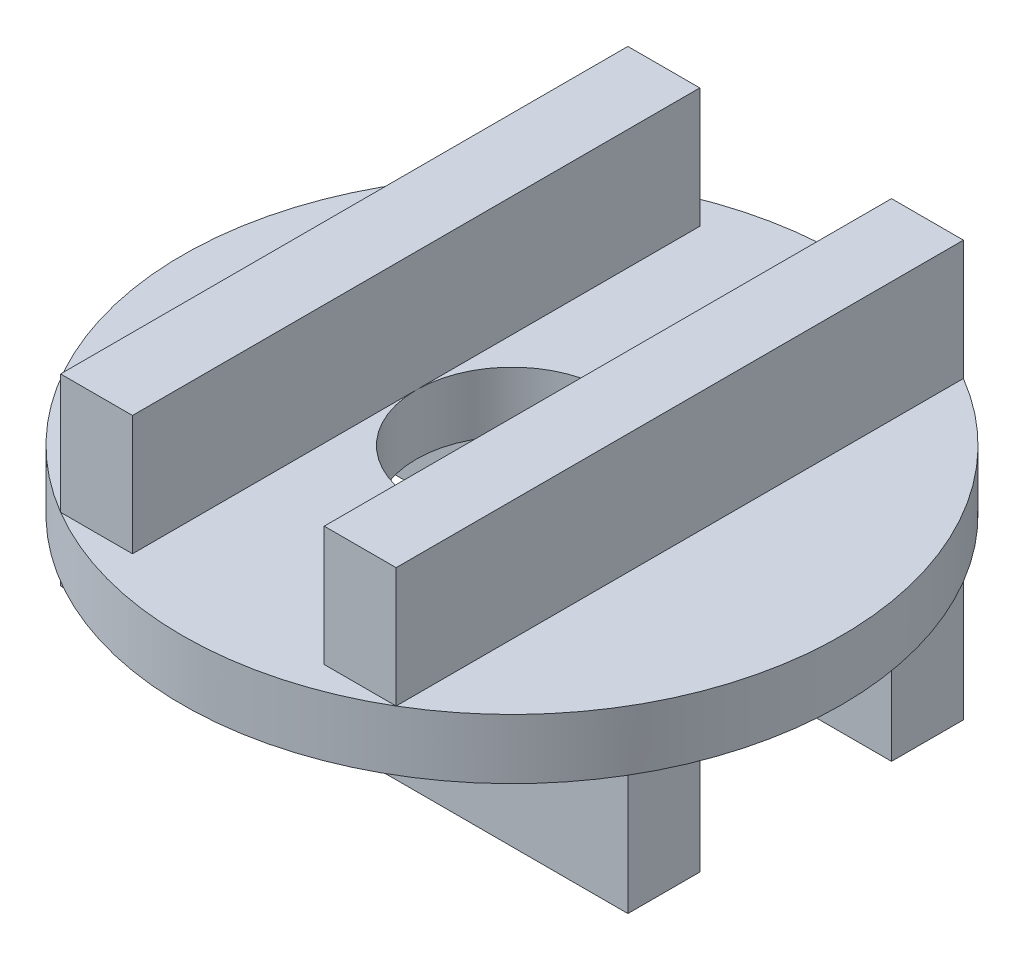
ISO-10303-21;
HEADER;
FILE_DESCRIPTION(('STEP AP214'),'2;1');
FILE_NAME('part.step','',(''),(''),'','','');
FILE_SCHEMA(('AUTOMOTIVE_DESIGN { 1 0 10303 214 1 1 1 1 }'));
ENDSEC;
DATA;
#1=APPLICATION_CONTEXT('core data for automotive mechanical design processes');
#2=APPLICATION_PROTOCOL_DEFINITION('international standard','automotive_design',2000,#1);
#3=PRODUCT_CONTEXT('',#1,'mechanical');
#4=PRODUCT('Part','Part','',(#3));
#5=PRODUCT_RELATED_PRODUCT_CATEGORY('part','',(#4));
#6=PRODUCT_DEFINITION_FORMATION('','',#4);
#7=PRODUCT_DEFINITION_CONTEXT('part definition',#1,'design');
#8=PRODUCT_DEFINITION('design','',#6,#7);
#9=PRODUCT_DEFINITION_SHAPE('','',#8);
#10=(LENGTH_UNIT() NAMED_UNIT(*) SI_UNIT(.MILLI.,.METRE.));
#11=(NAMED_UNIT(*) PLANE_ANGLE_UNIT() SI_UNIT($,.RADIAN.));
#12=(NAMED_UNIT(*) SI_UNIT($,.STERADIAN.) SOLID_ANGLE_UNIT());
#13=UNCERTAINTY_MEASURE_WITH_UNIT(LENGTH_MEASURE(1.E-05),#10,'distance_accuracy_value','');
#14=(GEOMETRIC_REPRESENTATION_CONTEXT(3) GLOBAL_UNCERTAINTY_ASSIGNED_CONTEXT((#13)) GLOBAL_UNIT_ASSIGNED_CONTEXT((#10,
#11,#12)) REPRESENTATION_CONTEXT('',''));
#15=CARTESIAN_POINT('',(0.,0.,0.));
#16=DIRECTION('',(0.,0.,1.));
#17=DIRECTION('',(1.,0.,0.));
#18=AXIS2_PLACEMENT_3D('',#15,#16,#17);
#19=CARTESIAN_POINT('',(0.,0.,0.));
#20=DIRECTION('',(0.,1.,0.));
#21=DIRECTION('',(0.,0.,1.));
#22=AXIS2_PLACEMENT_3D('',#19,#20,#21);
#23=PLANE('',#22);
#24=DIRECTION('',(0.,0.,1.));
#25=VECTOR('',#24,1.);
#26=CARTESIAN_POINT('',(47.3392015141785,0.,1.64240848401284E-13));
#27=LINE('',#26,#25);
#28=CARTESIAN_POINT('',(47.3392015141785,0.,16.0000000000002));
#29=VERTEX_POINT('',#28);
#30=CARTESIAN_POINT('',(47.3392015141784,0.,28.0000000000002));
#31=VERTEX_POINT('',#30);
#32=EDGE_CURVE('E70',#29,#31,#27,.T.);
#33=ORIENTED_EDGE('',*,*,#32,.F.);
#34=DIRECTION('',(-1.,0.,0.));
#35=VECTOR('',#34,1.);
#36=CARTESIAN_POINT('',(0.,0.,16.));
#37=LINE('',#36,#35);
#38=CARTESIAN_POINT('',(0.,0.,16.));
#39=VERTEX_POINT('',#38);
#40=EDGE_CURVE('E53',#29,#39,#37,.T.);
#41=ORIENTED_EDGE('',*,*,#40,.T.);
#42=CARTESIAN_POINT('',(0.,0.,0.));
#43=DIRECTION('',(0.,1.,0.));
#44=DIRECTION('',(0.,0.,1.));
#45=AXIS2_PLACEMENT_3D('',#42,#43,#44);
#46=CIRCLE('',#45,16.);
#47=CARTESIAN_POINT('',(0.,0.,-16.));
#48=VERTEX_POINT('',#47);
#49=EDGE_CURVE('E313',#39,#48,#46,.T.);
#50=ORIENTED_EDGE('',*,*,#49,.T.);
#51=DIRECTION('',(-1.,0.,0.));
#52=VECTOR('',#51,1.);
#53=CARTESIAN_POINT('',(0.,0.,-16.));
#54=LINE('',#53,#52);
#55=CARTESIAN_POINT('',(47.3392015141786,0.,-15.9999999999998));
#56=VERTEX_POINT('',#55);
#57=EDGE_CURVE('E228',#56,#48,#54,.T.);
#58=ORIENTED_EDGE('',*,*,#57,.F.);
#59=DIRECTION('',(0.,0.,-1.));
#60=VECTOR('',#59,1.);
#61=CARTESIAN_POINT('',(47.3392015141785,0.,1.64240848401285E-13));
#62=LINE('',#61,#60);
#63=CARTESIAN_POINT('',(47.3392015141786,0.,-27.9999999999998));
#64=VERTEX_POINT('',#63);
#65=EDGE_CURVE('E224',#56,#64,#62,.T.);
#66=ORIENTED_EDGE('',*,*,#65,.T.);
#67=CARTESIAN_POINT('',(0.,0.,0.));
#68=DIRECTION('',(0.,1.,0.));
#69=DIRECTION('',(0.,0.,1.));
#70=AXIS2_PLACEMENT_3D('',#67,#68,#69);
#71=CIRCLE('',#70,55.);
#72=EDGE_CURVE('E50',#31,#64,#71,.T.);
#73=ORIENTED_EDGE('',*,*,#72,.F.);
#74=EDGE_LOOP('',(#33,#41,#50,#58,#66,#73));
#75=FACE_BOUND('',#74,.T.);
#76=ADVANCED_FACE('F43',(#75),#23,.F.);
#77=DIRECTION('',(-1.,0.,0.));
#78=VECTOR('',#77,1.);
#79=CARTESIAN_POINT('',(0.,0.,28.));
#80=LINE('',#79,#78);
#81=CARTESIAN_POINT('',(-47.3392015141786,0.,27.9999999999998));
#82=VERTEX_POINT('',#81);
#83=EDGE_CURVE('E193',#31,#82,#80,.T.);
#84=ORIENTED_EDGE('',*,*,#83,.F.);
#85=EDGE_CURVE('E310',#82,#31,#71,.T.);
#86=ORIENTED_EDGE('',*,*,#85,.F.);
#87=EDGE_LOOP('',(#84,#86));
#88=FACE_BOUND('',#87,.T.);
#89=ADVANCED_FACE('F341',(#88),#23,.F.);
#90=EDGE_CURVE('E272',#48,#39,#46,.T.);
#91=ORIENTED_EDGE('',*,*,#90,.T.);
#92=CARTESIAN_POINT('',(-47.3392015141786,0.,15.9999999999998));
#93=VERTEX_POINT('',#92);
#94=EDGE_CURVE('E11',#39,#93,#37,.T.);
#95=ORIENTED_EDGE('',*,*,#94,.T.);
#96=DIRECTION('',(0.,0.,1.));
#97=VECTOR('',#96,1.);
#98=CARTESIAN_POINT('',(-47.3392015141785,0.,-1.64240848401284E-13));
#99=LINE('',#98,#97);
#100=EDGE_CURVE('E192',#93,#82,#99,.T.);
#101=ORIENTED_EDGE('',*,*,#100,.T.);
#102=CARTESIAN_POINT('',(-47.3392015141784,0.,-28.0000000000002));
#103=VERTEX_POINT('',#102);
#104=EDGE_CURVE('E332',#103,#82,#71,.T.);
#105=ORIENTED_EDGE('',*,*,#104,.F.);
#106=DIRECTION('',(0.,0.,-1.));
#107=VECTOR('',#106,1.);
#108=CARTESIAN_POINT('',(-47.3392015141785,0.,-1.91614323134832E-13));
#109=LINE('',#108,#107);
#110=CARTESIAN_POINT('',(-47.3392015141785,0.,-16.0000000000002));
#111=VERTEX_POINT('',#110);
#112=EDGE_CURVE('E215',#111,#103,#109,.T.);
#113=ORIENTED_EDGE('',*,*,#112,.F.);
#114=EDGE_CURVE('E55',#48,#111,#54,.T.);
#115=ORIENTED_EDGE('',*,*,#114,.F.);
#116=EDGE_LOOP('',(#91,#95,#101,#105,#113,#115));
#117=FACE_BOUND('',#116,.T.);
#118=ADVANCED_FACE('F350',(#117),#23,.F.);
#119=CARTESIAN_POINT('',(0.,10.,0.));
#120=DIRECTION('',(0.,1.,0.));
#121=DIRECTION('',(0.,0.,1.));
#122=AXIS2_PLACEMENT_3D('',#119,#120,#121);
#123=PLANE('',#122);
#124=DIRECTION('',(0.,0.,1.));
#125=VECTOR('',#124,1.);
#126=CARTESIAN_POINT('',(16.,10.,47.3392015141785));
#127=LINE('',#126,#125);
#128=CARTESIAN_POINT('',(16.,10.,0.));
#129=VERTEX_POINT('',#128);
#130=CARTESIAN_POINT('',(16.,10.,47.3392015141785));
#131=VERTEX_POINT('',#130);
#132=EDGE_CURVE('E261',#129,#131,#127,.T.);
#133=ORIENTED_EDGE('',*,*,#132,.F.);
#134=CARTESIAN_POINT('',(0.,10.,0.));
#135=DIRECTION('',(0.,1.,0.));
#136=DIRECTION('',(0.,0.,1.));
#137=AXIS2_PLACEMENT_3D('',#134,#135,#136);
#138=CIRCLE('',#137,16.);
#139=CARTESIAN_POINT('',(-16.,10.,0.));
#140=VERTEX_POINT('',#139);
#141=EDGE_CURVE('E309',#140,#129,#138,.T.);
#142=ORIENTED_EDGE('',*,*,#141,.F.);
#143=DIRECTION('',(0.,0.,-1.));
#144=VECTOR('',#143,1.);
#145=CARTESIAN_POINT('',(-16.,10.,47.3392015141785));
#146=LINE('',#145,#144);
#147=CARTESIAN_POINT('',(-16.,10.,47.3392015141785));
#148=VERTEX_POINT('',#147);
#149=EDGE_CURVE('E289',#148,#140,#146,.T.);
#150=ORIENTED_EDGE('',*,*,#149,.F.);
#151=DIRECTION('',(1.,0.,0.));
#152=VECTOR('',#151,1.);
#153=CARTESIAN_POINT('',(-16.,10.,47.3392015141785));
#154=LINE('',#153,#152);
#155=CARTESIAN_POINT('',(-28.,10.,47.3392015141785));
#156=VERTEX_POINT('',#155);
#157=EDGE_CURVE('E291',#156,#148,#154,.T.);
#158=ORIENTED_EDGE('',*,*,#157,.F.);
#159=CARTESIAN_POINT('',(0.,10.,0.));
#160=DIRECTION('',(0.,1.,0.));
#161=DIRECTION('',(0.,0.,1.));
#162=AXIS2_PLACEMENT_3D('',#159,#160,#161);
#163=CIRCLE('',#162,55.);
#164=CARTESIAN_POINT('',(28.,10.,47.3392015141785));
#165=VERTEX_POINT('',#164);
#166=EDGE_CURVE('E312',#156,#165,#163,.T.);
#167=ORIENTED_EDGE('',*,*,#166,.T.);
#168=DIRECTION('',(1.,0.,0.));
#169=VECTOR('',#168,1.);
#170=CARTESIAN_POINT('',(16.,10.,47.3392015141785));
#171=LINE('',#170,#169);
#172=EDGE_CURVE('E249',#131,#165,#171,.T.);
#173=ORIENTED_EDGE('',*,*,#172,.F.);
#174=EDGE_LOOP('',(#133,#142,#150,#158,#167,#173));
#175=FACE_BOUND('',#174,.T.);
#176=ADVANCED_FACE('F355',(#175),#123,.T.);
#177=CARTESIAN_POINT('',(16.,10.,-47.3392015141785));
#178=VERTEX_POINT('',#177);
#179=EDGE_CURVE('E245',#178,#129,#127,.T.);
#180=ORIENTED_EDGE('',*,*,#179,.F.);
#181=DIRECTION('',(-1.,0.,0.));
#182=VECTOR('',#181,1.);
#183=CARTESIAN_POINT('',(16.,10.,-47.3392015141785));
#184=LINE('',#183,#182);
#185=CARTESIAN_POINT('',(28.,10.,-47.3392015141785));
#186=VERTEX_POINT('',#185);
#187=EDGE_CURVE('E258',#186,#178,#184,.T.);
#188=ORIENTED_EDGE('',*,*,#187,.F.);
#189=CARTESIAN_POINT('',(-28.,10.,-47.3392015141785));
#190=VERTEX_POINT('',#189);
#191=EDGE_CURVE('E314',#186,#190,#163,.T.);
#192=ORIENTED_EDGE('',*,*,#191,.T.);
#193=DIRECTION('',(-1.,0.,0.));
#194=VECTOR('',#193,1.);
#195=CARTESIAN_POINT('',(-16.,10.,-47.3392015141785));
#196=LINE('',#195,#194);
#197=CARTESIAN_POINT('',(-16.,10.,-47.3392015141785));
#198=VERTEX_POINT('',#197);
#199=EDGE_CURVE('E287',#198,#190,#196,.T.);
#200=ORIENTED_EDGE('',*,*,#199,.F.);
#201=EDGE_CURVE('E294',#140,#198,#146,.T.);
#202=ORIENTED_EDGE('',*,*,#201,.F.);
#203=EDGE_CURVE('E308',#129,#140,#138,.T.);
#204=ORIENTED_EDGE('',*,*,#203,.F.);
#205=EDGE_LOOP('',(#180,#188,#192,#200,#202,#204));
#206=FACE_BOUND('',#205,.T.);
#207=ADVANCED_FACE('F589',(#206),#123,.T.);
#208=DIRECTION('',(0.,0.,-1.));
#209=VECTOR('',#208,1.);
#210=CARTESIAN_POINT('',(28.,10.,47.3392015141785));
#211=LINE('',#210,#209);
#212=EDGE_CURVE('E252',#165,#186,#211,.T.);
#213=ORIENTED_EDGE('',*,*,#212,.F.);
#214=EDGE_CURVE('E311',#165,#186,#163,.T.);
#215=ORIENTED_EDGE('',*,*,#214,.T.);
#216=EDGE_LOOP('',(#213,#215));
#217=FACE_BOUND('',#216,.T.);
#218=ADVANCED_FACE('F356',(#217),#123,.T.);
#219=DIRECTION('',(0.,0.,1.));
#220=VECTOR('',#219,1.);
#221=CARTESIAN_POINT('',(-28.,10.,47.3392015141785));
#222=LINE('',#221,#220);
#223=EDGE_CURVE('E251',#190,#156,#222,.T.);
#224=ORIENTED_EDGE('',*,*,#223,.F.);
#225=EDGE_CURVE('E321',#190,#156,#163,.T.);
#226=ORIENTED_EDGE('',*,*,#225,.T.);
#227=EDGE_LOOP('',(#224,#226));
#228=FACE_BOUND('',#227,.T.);
#229=ADVANCED_FACE('F357',(#228),#123,.T.);
#230=EDGE_CURVE('E330',#64,#103,#71,.T.);
#231=ORIENTED_EDGE('',*,*,#230,.F.);
#232=DIRECTION('',(-1.,0.,0.));
#233=VECTOR('',#232,1.);
#234=CARTESIAN_POINT('',(0.,0.,-28.));
#235=LINE('',#234,#233);
#236=EDGE_CURVE('E219',#64,#103,#235,.T.);
#237=ORIENTED_EDGE('',*,*,#236,.T.);
#238=EDGE_LOOP('',(#231,#237));
#239=FACE_BOUND('',#238,.T.);
#240=ADVANCED_FACE('F351',(#239),#23,.F.);
#241=CARTESIAN_POINT('',(0.,10.,0.));
#242=DIRECTION('',(0.,-1.,0.));
#243=DIRECTION('',(0.,0.,-1.));
#244=AXIS2_PLACEMENT_3D('',#241,#242,#243);
#245=CYLINDRICAL_SURFACE('',#244,55.);
#246=ORIENTED_EDGE('',*,*,#214,.F.);
#247=ORIENTED_EDGE('',*,*,#166,.F.);
#248=ORIENTED_EDGE('',*,*,#225,.F.);
#249=ORIENTED_EDGE('',*,*,#191,.F.);
#250=EDGE_LOOP('',(#246,#247,#248,#249));
#251=FACE_BOUND('',#250,.T.);
#252=ORIENTED_EDGE('',*,*,#72,.T.);
#253=ORIENTED_EDGE('',*,*,#230,.T.);
#254=ORIENTED_EDGE('',*,*,#104,.T.);
#255=ORIENTED_EDGE('',*,*,#85,.T.);
#256=EDGE_LOOP('',(#252,#253,#254,#255));
#257=FACE_BOUND('',#256,.T.);
#258=ADVANCED_FACE('F44',(#251,#257),#245,.T.);
#259=CARTESIAN_POINT('',(0.,10.,0.));
#260=DIRECTION('',(0.,-1.,0.));
#261=DIRECTION('',(0.,0.,-1.));
#262=AXIS2_PLACEMENT_3D('',#259,#260,#261);
#263=CYLINDRICAL_SURFACE('',#262,16.);
#264=ORIENTED_EDGE('',*,*,#203,.T.);
#265=ORIENTED_EDGE('',*,*,#141,.T.);
#266=EDGE_LOOP('',(#264,#265));
#267=FACE_BOUND('',#266,.T.);
#268=ORIENTED_EDGE('',*,*,#49,.F.);
#269=ORIENTED_EDGE('',*,*,#90,.F.);
#270=EDGE_LOOP('',(#268,#269));
#271=FACE_BOUND('',#270,.T.);
#272=ADVANCED_FACE('F362',(#267,#271),#263,.F.);
#273=CARTESIAN_POINT('',(-28.,30.,47.3392015141785));
#274=DIRECTION('',(1.,0.,0.));
#275=DIRECTION('',(0.,0.,-1.));
#276=AXIS2_PLACEMENT_3D('',#273,#274,#275);
#277=PLANE('',#276);
#278=ORIENTED_EDGE('',*,*,#223,.T.);
#279=DIRECTION('',(0.,-1.,0.));
#280=VECTOR('',#279,1.);
#281=CARTESIAN_POINT('',(-28.,30.,47.3392015141785));
#282=LINE('',#281,#280);
#283=CARTESIAN_POINT('',(-28.,30.,47.3392015141785));
#284=VERTEX_POINT('',#283);
#285=EDGE_CURVE('E180',#284,#156,#282,.T.);
#286=ORIENTED_EDGE('',*,*,#285,.F.);
#287=DIRECTION('',(0.,0.,1.));
#288=VECTOR('',#287,1.);
#289=CARTESIAN_POINT('',(-28.,30.,47.3392015141785));
#290=LINE('',#289,#288);
#291=CARTESIAN_POINT('',(-28.,30.,-47.3392015141785));
#292=VERTEX_POINT('',#291);
#293=EDGE_CURVE('E286',#292,#284,#290,.T.);
#294=ORIENTED_EDGE('',*,*,#293,.F.);
#295=DIRECTION('',(0.,-1.,0.));
#296=VECTOR('',#295,1.);
#297=CARTESIAN_POINT('',(-28.,30.,-47.3392015141785));
#298=LINE('',#297,#296);
#299=EDGE_CURVE('E285',#292,#190,#298,.T.);
#300=ORIENTED_EDGE('',*,*,#299,.T.);
#301=EDGE_LOOP('',(#278,#286,#294,#300));
#302=FACE_BOUND('',#301,.T.);
#303=ADVANCED_FACE('F364',(#302),#277,.F.);
#304=CARTESIAN_POINT('',(-16.,30.,47.3392015141785));
#305=DIRECTION('',(0.,0.,-1.));
#306=DIRECTION('',(-1.,0.,0.));
#307=AXIS2_PLACEMENT_3D('',#304,#305,#306);
#308=PLANE('',#307);
#309=ORIENTED_EDGE('',*,*,#157,.T.);
#310=DIRECTION('',(0.,-1.,0.));
#311=VECTOR('',#310,1.);
#312=CARTESIAN_POINT('',(-16.,30.,47.3392015141785));
#313=LINE('',#312,#311);
#314=CARTESIAN_POINT('',(-16.,30.,47.3392015141785));
#315=VERTEX_POINT('',#314);
#316=EDGE_CURVE('E277',#315,#148,#313,.T.);
#317=ORIENTED_EDGE('',*,*,#316,.F.);
#318=DIRECTION('',(1.,0.,0.));
#319=VECTOR('',#318,1.);
#320=CARTESIAN_POINT('',(-16.,30.,47.3392015141785));
#321=LINE('',#320,#319);
#322=EDGE_CURVE('E305',#284,#315,#321,.T.);
#323=ORIENTED_EDGE('',*,*,#322,.F.);
#324=ORIENTED_EDGE('',*,*,#285,.T.);
#325=EDGE_LOOP('',(#309,#317,#323,#324));
#326=FACE_BOUND('',#325,.T.);
#327=ADVANCED_FACE('F377',(#326),#308,.F.);
#328=CARTESIAN_POINT('',(-16.,30.,47.3392015141785));
#329=DIRECTION('',(-1.,0.,0.));
#330=DIRECTION('',(0.,0.,1.));
#331=AXIS2_PLACEMENT_3D('',#328,#329,#330);
#332=PLANE('',#331);
#333=ORIENTED_EDGE('',*,*,#149,.T.);
#334=ORIENTED_EDGE('',*,*,#201,.T.);
#335=DIRECTION('',(0.,-1.,0.));
#336=VECTOR('',#335,1.);
#337=CARTESIAN_POINT('',(-16.,30.,-47.3392015141785));
#338=LINE('',#337,#336);
#339=CARTESIAN_POINT('',(-16.,30.,-47.3392015141785));
#340=VERTEX_POINT('',#339);
#341=EDGE_CURVE('E276',#340,#198,#338,.T.);
#342=ORIENTED_EDGE('',*,*,#341,.F.);
#343=DIRECTION('',(0.,0.,-1.));
#344=VECTOR('',#343,1.);
#345=CARTESIAN_POINT('',(-16.,30.,47.3392015141785));
#346=LINE('',#345,#344);
#347=EDGE_CURVE('E297',#315,#340,#346,.T.);
#348=ORIENTED_EDGE('',*,*,#347,.F.);
#349=ORIENTED_EDGE('',*,*,#316,.T.);
#350=EDGE_LOOP('',(#333,#334,#342,#348,#349));
#351=FACE_BOUND('',#350,.T.);
#352=ADVANCED_FACE('F374',(#351),#332,.F.);
#353=CARTESIAN_POINT('',(-16.,30.,-47.3392015141785));
#354=DIRECTION('',(0.,0.,1.));
#355=DIRECTION('',(1.,0.,0.));
#356=AXIS2_PLACEMENT_3D('',#353,#354,#355);
#357=PLANE('',#356);
#358=ORIENTED_EDGE('',*,*,#199,.T.);
#359=ORIENTED_EDGE('',*,*,#299,.F.);
#360=DIRECTION('',(-1.,0.,0.));
#361=VECTOR('',#360,1.);
#362=CARTESIAN_POINT('',(-16.,30.,-47.3392015141785));
#363=LINE('',#362,#361);
#364=EDGE_CURVE('E282',#340,#292,#363,.T.);
#365=ORIENTED_EDGE('',*,*,#364,.F.);
#366=ORIENTED_EDGE('',*,*,#341,.T.);
#367=EDGE_LOOP('',(#358,#359,#365,#366));
#368=FACE_BOUND('',#367,.T.);
#369=ADVANCED_FACE('F371',(#368),#357,.F.);
#370=CARTESIAN_POINT('',(0.,30.,0.));
#371=DIRECTION('',(0.,1.,0.));
#372=DIRECTION('',(0.,0.,1.));
#373=AXIS2_PLACEMENT_3D('',#370,#371,#372);
#374=PLANE('',#373);
#375=ORIENTED_EDGE('',*,*,#293,.T.);
#376=ORIENTED_EDGE('',*,*,#322,.T.);
#377=ORIENTED_EDGE('',*,*,#347,.T.);
#378=ORIENTED_EDGE('',*,*,#364,.T.);
#379=EDGE_LOOP('',(#375,#376,#377,#378));
#380=FACE_BOUND('',#379,.T.);
#381=ADVANCED_FACE('F370',(#380),#374,.T.);
#382=CARTESIAN_POINT('',(16.,30.,47.3392015141785));
#383=DIRECTION('',(0.,0.,-1.));
#384=DIRECTION('',(-1.,0.,0.));
#385=AXIS2_PLACEMENT_3D('',#382,#383,#384);
#386=PLANE('',#385);
#387=ORIENTED_EDGE('',*,*,#172,.T.);
#388=DIRECTION('',(0.,-1.,0.));
#389=VECTOR('',#388,1.);
#390=CARTESIAN_POINT('',(28.,30.,47.3392015141785));
#391=LINE('',#390,#389);
#392=CARTESIAN_POINT('',(28.,30.,47.3392015141785));
#393=VERTEX_POINT('',#392);
#394=EDGE_CURVE('E269',#393,#165,#391,.T.);
#395=ORIENTED_EDGE('',*,*,#394,.F.);
#396=DIRECTION('',(1.,0.,0.));
#397=VECTOR('',#396,1.);
#398=CARTESIAN_POINT('',(16.,30.,47.3392015141785));
#399=LINE('',#398,#397);
#400=CARTESIAN_POINT('',(16.,30.,47.3392015141785));
#401=VERTEX_POINT('',#400);
#402=EDGE_CURVE('E236',#401,#393,#399,.T.);
#403=ORIENTED_EDGE('',*,*,#402,.F.);
#404=DIRECTION('',(0.,-1.,0.));
#405=VECTOR('',#404,1.);
#406=CARTESIAN_POINT('',(16.,30.,47.3392015141785));
#407=LINE('',#406,#405);
#408=EDGE_CURVE('E248',#401,#131,#407,.T.);
#409=ORIENTED_EDGE('',*,*,#408,.T.);
#410=EDGE_LOOP('',(#387,#395,#403,#409));
#411=FACE_BOUND('',#410,.T.);
#412=ADVANCED_FACE('F367',(#411),#386,.F.);
#413=CARTESIAN_POINT('',(28.,30.,47.3392015141785));
#414=DIRECTION('',(-1.,0.,0.));
#415=DIRECTION('',(0.,0.,1.));
#416=AXIS2_PLACEMENT_3D('',#413,#414,#415);
#417=PLANE('',#416);
#418=ORIENTED_EDGE('',*,*,#212,.T.);
#419=DIRECTION('',(0.,-1.,0.));
#420=VECTOR('',#419,1.);
#421=CARTESIAN_POINT('',(28.,30.,-47.3392015141785));
#422=LINE('',#421,#420);
#423=CARTESIAN_POINT('',(28.,30.,-47.3392015141785));
#424=VERTEX_POINT('',#423);
#425=EDGE_CURVE('E270',#424,#186,#422,.T.);
#426=ORIENTED_EDGE('',*,*,#425,.F.);
#427=DIRECTION('',(0.,0.,-1.));
#428=VECTOR('',#427,1.);
#429=CARTESIAN_POINT('',(28.,30.,47.3392015141785));
#430=LINE('',#429,#428);
#431=EDGE_CURVE('E243',#393,#424,#430,.T.);
#432=ORIENTED_EDGE('',*,*,#431,.F.);
#433=ORIENTED_EDGE('',*,*,#394,.T.);
#434=EDGE_LOOP('',(#418,#426,#432,#433));
#435=FACE_BOUND('',#434,.T.);
#436=ADVANCED_FACE('F386',(#435),#417,.F.);
#437=CARTESIAN_POINT('',(16.,30.,-47.3392015141785));
#438=DIRECTION('',(0.,0.,1.));
#439=DIRECTION('',(1.,0.,0.));
#440=AXIS2_PLACEMENT_3D('',#437,#438,#439);
#441=PLANE('',#440);
#442=ORIENTED_EDGE('',*,*,#187,.T.);
#443=DIRECTION('',(0.,-1.,0.));
#444=VECTOR('',#443,1.);
#445=CARTESIAN_POINT('',(16.,30.,-47.3392015141785));
#446=LINE('',#445,#444);
#447=CARTESIAN_POINT('',(16.,30.,-47.3392015141785));
#448=VERTEX_POINT('',#447);
#449=EDGE_CURVE('E262',#448,#178,#446,.T.);
#450=ORIENTED_EDGE('',*,*,#449,.F.);
#451=DIRECTION('',(-1.,0.,0.));
#452=VECTOR('',#451,1.);
#453=CARTESIAN_POINT('',(16.,30.,-47.3392015141785));
#454=LINE('',#453,#452);
#455=EDGE_CURVE('E244',#424,#448,#454,.T.);
#456=ORIENTED_EDGE('',*,*,#455,.F.);
#457=ORIENTED_EDGE('',*,*,#425,.T.);
#458=EDGE_LOOP('',(#442,#450,#456,#457));
#459=FACE_BOUND('',#458,.T.);
#460=ADVANCED_FACE('F391',(#459),#441,.F.);
#461=CARTESIAN_POINT('',(16.,30.,47.3392015141785));
#462=DIRECTION('',(1.,0.,0.));
#463=DIRECTION('',(0.,0.,-1.));
#464=AXIS2_PLACEMENT_3D('',#461,#462,#463);
#465=PLANE('',#464);
#466=ORIENTED_EDGE('',*,*,#179,.T.);
#467=ORIENTED_EDGE('',*,*,#132,.T.);
#468=ORIENTED_EDGE('',*,*,#408,.F.);
#469=DIRECTION('',(0.,0.,1.));
#470=VECTOR('',#469,1.);
#471=CARTESIAN_POINT('',(16.,30.,47.3392015141785));
#472=LINE('',#471,#470);
#473=EDGE_CURVE('E247',#448,#401,#472,.T.);
#474=ORIENTED_EDGE('',*,*,#473,.F.);
#475=ORIENTED_EDGE('',*,*,#449,.T.);
#476=EDGE_LOOP('',(#466,#467,#468,#474,#475));
#477=FACE_BOUND('',#476,.T.);
#478=ADVANCED_FACE('F400',(#477),#465,.F.);
#479=CARTESIAN_POINT('',(0.,30.,0.));
#480=DIRECTION('',(0.,1.,0.));
#481=DIRECTION('',(0.,0.,1.));
#482=AXIS2_PLACEMENT_3D('',#479,#480,#481);
#483=PLANE('',#482);
#484=ORIENTED_EDGE('',*,*,#402,.T.);
#485=ORIENTED_EDGE('',*,*,#431,.T.);
#486=ORIENTED_EDGE('',*,*,#455,.T.);
#487=ORIENTED_EDGE('',*,*,#473,.T.);
#488=EDGE_LOOP('',(#484,#485,#486,#487));
#489=FACE_BOUND('',#488,.T.);
#490=ADVANCED_FACE('F402',(#489),#483,.T.);
#491=CARTESIAN_POINT('',(0.,-20.,-28.));
#492=DIRECTION('',(0.,0.,-1.));
#493=DIRECTION('',(-1.,0.,0.));
#494=AXIS2_PLACEMENT_3D('',#491,#492,#493);
#495=PLANE('',#494);
#496=ORIENTED_EDGE('',*,*,#236,.F.);
#497=DIRECTION('',(0.,1.,0.));
#498=VECTOR('',#497,1.);
#499=CARTESIAN_POINT('',(47.3392015141786,-20.,-27.9999999999998));
#500=LINE('',#499,#498);
#501=CARTESIAN_POINT('',(47.3392015141786,-20.,-27.9999999999998));
#502=VERTEX_POINT('',#501);
#503=EDGE_CURVE('E200',#502,#64,#500,.T.);
#504=ORIENTED_EDGE('',*,*,#503,.F.);
#505=DIRECTION('',(-1.,0.,0.));
#506=VECTOR('',#505,1.);
#507=CARTESIAN_POINT('',(0.,-20.,-28.));
#508=LINE('',#507,#506);
#509=CARTESIAN_POINT('',(-47.3392015141784,-20.,-28.0000000000002));
#510=VERTEX_POINT('',#509);
#511=EDGE_CURVE('E208',#502,#510,#508,.T.);
#512=ORIENTED_EDGE('',*,*,#511,.T.);
#513=DIRECTION('',(0.,1.,0.));
#514=VECTOR('',#513,1.);
#515=CARTESIAN_POINT('',(-47.3392015141784,-20.,-28.0000000000002));
#516=LINE('',#515,#514);
#517=EDGE_CURVE('E218',#510,#103,#516,.T.);
#518=ORIENTED_EDGE('',*,*,#517,.T.);
#519=EDGE_LOOP('',(#496,#504,#512,#518));
#520=FACE_BOUND('',#519,.T.);
#521=ADVANCED_FACE('F403',(#520),#495,.T.);
#522=CARTESIAN_POINT('',(47.3392015141785,-20.,1.64240848401285E-13));
#523=DIRECTION('',(1.,0.,0.));
#524=DIRECTION('',(0.,0.,-1.));
#525=AXIS2_PLACEMENT_3D('',#522,#523,#524);
#526=PLANE('',#525);
#527=ORIENTED_EDGE('',*,*,#65,.F.);
#528=DIRECTION('',(0.,1.,0.));
#529=VECTOR('',#528,1.);
#530=CARTESIAN_POINT('',(47.3392015141786,-20.,-15.9999999999998));
#531=LINE('',#530,#529);
#532=CARTESIAN_POINT('',(47.3392015141786,-20.,-15.9999999999998));
#533=VERTEX_POINT('',#532);
#534=EDGE_CURVE('E234',#533,#56,#531,.T.);
#535=ORIENTED_EDGE('',*,*,#534,.F.);
#536=DIRECTION('',(0.,0.,-1.));
#537=VECTOR('',#536,1.);
#538=CARTESIAN_POINT('',(47.3392015141785,-20.,1.64240848401285E-13));
#539=LINE('',#538,#537);
#540=EDGE_CURVE('E211',#533,#502,#539,.T.);
#541=ORIENTED_EDGE('',*,*,#540,.T.);
#542=ORIENTED_EDGE('',*,*,#503,.T.);
#543=EDGE_LOOP('',(#527,#535,#541,#542));
#544=FACE_BOUND('',#543,.T.);
#545=ADVANCED_FACE('F409',(#544),#526,.T.);
#546=CARTESIAN_POINT('',(0.,-20.,-16.));
#547=DIRECTION('',(0.,0.,-1.));
#548=DIRECTION('',(-1.,0.,0.));
#549=AXIS2_PLACEMENT_3D('',#546,#547,#548);
#550=PLANE('',#549);
#551=ORIENTED_EDGE('',*,*,#57,.T.);
#552=ORIENTED_EDGE('',*,*,#114,.T.);
#553=DIRECTION('',(0.,1.,0.));
#554=VECTOR('',#553,1.);
#555=CARTESIAN_POINT('',(-47.3392015141785,-20.,-16.0000000000002));
#556=LINE('',#555,#554);
#557=CARTESIAN_POINT('',(-47.3392015141785,-20.,-16.0000000000002));
#558=VERTEX_POINT('',#557);
#559=EDGE_CURVE('E232',#558,#111,#556,.T.);
#560=ORIENTED_EDGE('',*,*,#559,.F.);
#561=DIRECTION('',(-1.,0.,0.));
#562=VECTOR('',#561,1.);
#563=CARTESIAN_POINT('',(0.,-20.,-16.));
#564=LINE('',#563,#562);
#565=EDGE_CURVE('E214',#533,#558,#564,.T.);
#566=ORIENTED_EDGE('',*,*,#565,.F.);
#567=ORIENTED_EDGE('',*,*,#534,.T.);
#568=EDGE_LOOP('',(#551,#552,#560,#566,#567));
#569=FACE_BOUND('',#568,.T.);
#570=ADVANCED_FACE('F413',(#569),#550,.F.);
#571=CARTESIAN_POINT('',(-47.3392015141785,-20.,-1.91614323134832E-13));
#572=DIRECTION('',(1.,0.,0.));
#573=DIRECTION('',(0.,0.,-1.));
#574=AXIS2_PLACEMENT_3D('',#571,#572,#573);
#575=PLANE('',#574);
#576=ORIENTED_EDGE('',*,*,#112,.T.);
#577=ORIENTED_EDGE('',*,*,#517,.F.);
#578=DIRECTION('',(0.,0.,-1.));
#579=VECTOR('',#578,1.);
#580=CARTESIAN_POINT('',(-47.3392015141785,-20.,-1.91614323134832E-13));
#581=LINE('',#580,#579);
#582=EDGE_CURVE('E220',#558,#510,#581,.T.);
#583=ORIENTED_EDGE('',*,*,#582,.F.);
#584=ORIENTED_EDGE('',*,*,#559,.T.);
#585=EDGE_LOOP('',(#576,#577,#583,#584));
#586=FACE_BOUND('',#585,.T.);
#587=ADVANCED_FACE('F417',(#586),#575,.F.);
#588=CARTESIAN_POINT('',(0.,-20.,0.));
#589=DIRECTION('',(0.,-1.,0.));
#590=DIRECTION('',(0.,0.,-1.));
#591=AXIS2_PLACEMENT_3D('',#588,#589,#590);
#592=PLANE('',#591);
#593=ORIENTED_EDGE('',*,*,#511,.F.);
#594=ORIENTED_EDGE('',*,*,#540,.F.);
#595=ORIENTED_EDGE('',*,*,#565,.T.);
#596=ORIENTED_EDGE('',*,*,#582,.T.);
#597=EDGE_LOOP('',(#593,#594,#595,#596));
#598=FACE_BOUND('',#597,.T.);
#599=ADVANCED_FACE('F423',(#598),#592,.T.);
#600=CARTESIAN_POINT('',(0.,-20.,16.));
#601=DIRECTION('',(0.,0.,-1.));
#602=DIRECTION('',(-1.,0.,0.));
#603=AXIS2_PLACEMENT_3D('',#600,#601,#602);
#604=PLANE('',#603);
#605=ORIENTED_EDGE('',*,*,#40,.F.);
#606=DIRECTION('',(0.,1.,0.));
#607=VECTOR('',#606,1.);
#608=CARTESIAN_POINT('',(47.3392015141785,-20.,16.0000000000002));
#609=LINE('',#608,#607);
#610=CARTESIAN_POINT('',(47.3392015141785,-20.,16.0000000000002));
#611=VERTEX_POINT('',#610);
#612=EDGE_CURVE('E168',#611,#29,#609,.T.);
#613=ORIENTED_EDGE('',*,*,#612,.F.);
#614=DIRECTION('',(-1.,0.,0.));
#615=VECTOR('',#614,1.);
#616=CARTESIAN_POINT('',(0.,-20.,16.));
#617=LINE('',#616,#615);
#618=CARTESIAN_POINT('',(-47.3392015141786,-20.,15.9999999999998));
#619=VERTEX_POINT('',#618);
#620=EDGE_CURVE('E174',#611,#619,#617,.T.);
#621=ORIENTED_EDGE('',*,*,#620,.T.);
#622=DIRECTION('',(0.,1.,0.));
#623=VECTOR('',#622,1.);
#624=CARTESIAN_POINT('',(-47.3392015141786,-20.,15.9999999999998));
#625=LINE('',#624,#623);
#626=EDGE_CURVE('E197',#619,#93,#625,.T.);
#627=ORIENTED_EDGE('',*,*,#626,.T.);
#628=ORIENTED_EDGE('',*,*,#94,.F.);
#629=EDGE_LOOP('',(#605,#613,#621,#627,#628));
#630=FACE_BOUND('',#629,.T.);
#631=ADVANCED_FACE('F175',(#630),#604,.T.);
#632=CARTESIAN_POINT('',(47.3392015141785,-20.,1.64240848401284E-13));
#633=DIRECTION('',(-1.,0.,0.));
#634=DIRECTION('',(0.,0.,1.));
#635=AXIS2_PLACEMENT_3D('',#632,#633,#634);
#636=PLANE('',#635);
#637=ORIENTED_EDGE('',*,*,#32,.T.);
#638=DIRECTION('',(0.,1.,0.));
#639=VECTOR('',#638,1.);
#640=CARTESIAN_POINT('',(47.3392015141784,-20.,28.0000000000002));
#641=LINE('',#640,#639);
#642=CARTESIAN_POINT('',(47.3392015141784,-20.,28.0000000000002));
#643=VERTEX_POINT('',#642);
#644=EDGE_CURVE('E178',#643,#31,#641,.T.);
#645=ORIENTED_EDGE('',*,*,#644,.F.);
#646=DIRECTION('',(0.,0.,1.));
#647=VECTOR('',#646,1.);
#648=CARTESIAN_POINT('',(47.3392015141785,-20.,1.64240848401284E-13));
#649=LINE('',#648,#647);
#650=EDGE_CURVE('E182',#611,#643,#649,.T.);
#651=ORIENTED_EDGE('',*,*,#650,.F.);
#652=ORIENTED_EDGE('',*,*,#612,.T.);
#653=EDGE_LOOP('',(#637,#645,#651,#652));
#654=FACE_BOUND('',#653,.T.);
#655=ADVANCED_FACE('F185',(#654),#636,.F.);
#656=CARTESIAN_POINT('',(0.,-20.,28.));
#657=DIRECTION('',(0.,0.,-1.));
#658=DIRECTION('',(-1.,0.,0.));
#659=AXIS2_PLACEMENT_3D('',#656,#657,#658);
#660=PLANE('',#659);
#661=ORIENTED_EDGE('',*,*,#83,.T.);
#662=DIRECTION('',(0.,1.,0.));
#663=VECTOR('',#662,1.);
#664=CARTESIAN_POINT('',(-47.3392015141786,-20.,27.9999999999998));
#665=LINE('',#664,#663);
#666=CARTESIAN_POINT('',(-47.3392015141786,-20.,27.9999999999998));
#667=VERTEX_POINT('',#666);
#668=EDGE_CURVE('E204',#667,#82,#665,.T.);
#669=ORIENTED_EDGE('',*,*,#668,.F.);
#670=DIRECTION('',(-1.,0.,0.));
#671=VECTOR('',#670,1.);
#672=CARTESIAN_POINT('',(0.,-20.,28.));
#673=LINE('',#672,#671);
#674=EDGE_CURVE('E188',#643,#667,#673,.T.);
#675=ORIENTED_EDGE('',*,*,#674,.F.);
#676=ORIENTED_EDGE('',*,*,#644,.T.);
#677=EDGE_LOOP('',(#661,#669,#675,#676));
#678=FACE_BOUND('',#677,.T.);
#679=ADVANCED_FACE('F343',(#678),#660,.F.);
#680=CARTESIAN_POINT('',(-47.3392015141785,-20.,-1.64240848401284E-13));
#681=DIRECTION('',(-1.,0.,0.));
#682=DIRECTION('',(0.,0.,1.));
#683=AXIS2_PLACEMENT_3D('',#680,#681,#682);
#684=PLANE('',#683);
#685=ORIENTED_EDGE('',*,*,#100,.F.);
#686=ORIENTED_EDGE('',*,*,#626,.F.);
#687=DIRECTION('',(0.,0.,1.));
#688=VECTOR('',#687,1.);
#689=CARTESIAN_POINT('',(-47.3392015141785,-20.,-1.64240848401284E-13));
#690=LINE('',#689,#688);
#691=EDGE_CURVE('E187',#619,#667,#690,.T.);
#692=ORIENTED_EDGE('',*,*,#691,.T.);
#693=ORIENTED_EDGE('',*,*,#668,.T.);
#694=EDGE_LOOP('',(#685,#686,#692,#693));
#695=FACE_BOUND('',#694,.T.);
#696=ADVANCED_FACE('F342',(#695),#684,.T.);
#697=CARTESIAN_POINT('',(0.,-20.,0.));
#698=DIRECTION('',(0.,-1.,0.));
#699=DIRECTION('',(0.,0.,-1.));
#700=AXIS2_PLACEMENT_3D('',#697,#698,#699);
#701=PLANE('',#700);
#702=ORIENTED_EDGE('',*,*,#620,.F.);
#703=ORIENTED_EDGE('',*,*,#650,.T.);
#704=ORIENTED_EDGE('',*,*,#674,.T.);
#705=ORIENTED_EDGE('',*,*,#691,.F.);
#706=EDGE_LOOP('',(#702,#703,#704,#705));
#707=FACE_BOUND('',#706,.T.);
#708=ADVANCED_FACE('F186',(#707),#701,.T.);
#709=CLOSED_SHELL('',(#76,#89,#118,#176,#207,#218,#229,#240,#258,#272,#303,#327,#352,#369,#381,
#412,#436,#460,#478,#490,#521,#545,#570,#587,#599,#631,#655,#679,#696,#708));
#710=MANIFOLD_SOLID_BREP('B2',#709);
#711=ADVANCED_BREP_SHAPE_REPRESENTATION('',(#18,#710),#14);
#712=SHAPE_DEFINITION_REPRESENTATION(#9,#711);
ENDSEC;
END-ISO-10303-21;
